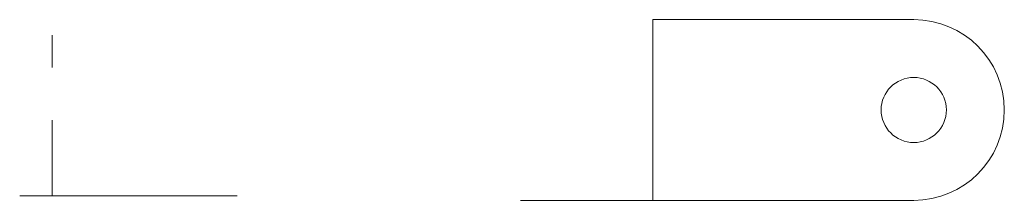
# Model space of a CAD drawing. Units: millimetres. Extents: x 201 to 472, y -1 to 49.
import ezdxf

# ---------------------------------------------------------------- set-up
doc = ezdxf.new("R2010")
doc.units = ezdxf.units.MM
doc.layers.add('M-CONS', color=8, linetype='Continuous', lineweight=13)

msp = doc.modelspace()

# ---------------------------------------------------------------- linework, layer by layer
at = {"layer": 'M-CONS'}
for p, q in [((209.65, 21, 61.95), (209.65, 0, 61.95)), ((447.39, -1.21), (415.39, -1.21)), ((415.39, -1.21, -18), (447.39, -1.21, -18))]:
    msp.add_line(p, q, dxfattribs=at)
at = {"layer": 'M-CONS', "extrusion": (0, -1, 0)}
msp.add_line((209.65, 0, 61.95), (209.65, 0, 81.95), dxfattribs=at)
at = {"layer": 'M-CONS'}
msp.add_lwpolyline([(447.39, -1.21, 1), (447.39, 48.79), (375.39, 48.79), (375.39, -1.21)], format="xyb", close=True, dxfattribs=at)
at = {"layer": 'M-CONS', "extrusion": (1, 0, 0), "elevation": 375.39}
msp.add_lwpolyline([(48.79, 16), (48.79, 26, 0.414214), (38.79, 36), (8.79, 36, 0.414214), (-1.21, 26), (-1.21, 16)], format="xyb", close=True, dxfattribs=at)
at = {"layer": 'M-CONS', "extrusion": (0, -1, 0)}
msp.add_lwpolyline([(239.65, 49.95), (239.65, 52.95), (260.65, 52.95), (260.65, 61.95), (200.65, 61.95), (200.65, 49.95)], close=True, dxfattribs=at)
at = {"layer": 'M-CONS', "extrusion": (0, -1, 0), "elevation": 1.21}
msp.add_lwpolyline([(362.39, 5.97), (362.39, 16, 33.303306), (365.39, 16), (365.39, 5.97, -19.949874)], format="xyb", close=True, dxfattribs=at)
at = {"layer": 'M-CONS', "extrusion": (1, 0, -1e-16)}
for centre in [(40, 81.95, 209.65), (10, 81.95, 209.65)]:
    msp.add_circle(centre, 4.5, dxfattribs=at)
at = {"layer": 'M-CONS', "extrusion": (1, 0, 0)}
for centre in [(36.29, 26, 375.39), (11.29, 26, 375.39)]:
    msp.add_circle(centre, 5, dxfattribs=at)
at = {"layer": 'M-CONS'}
msp.add_circle((447.39, 23.79, 16), 9, dxfattribs=at)

doc.saveas('drawing.dxf')
